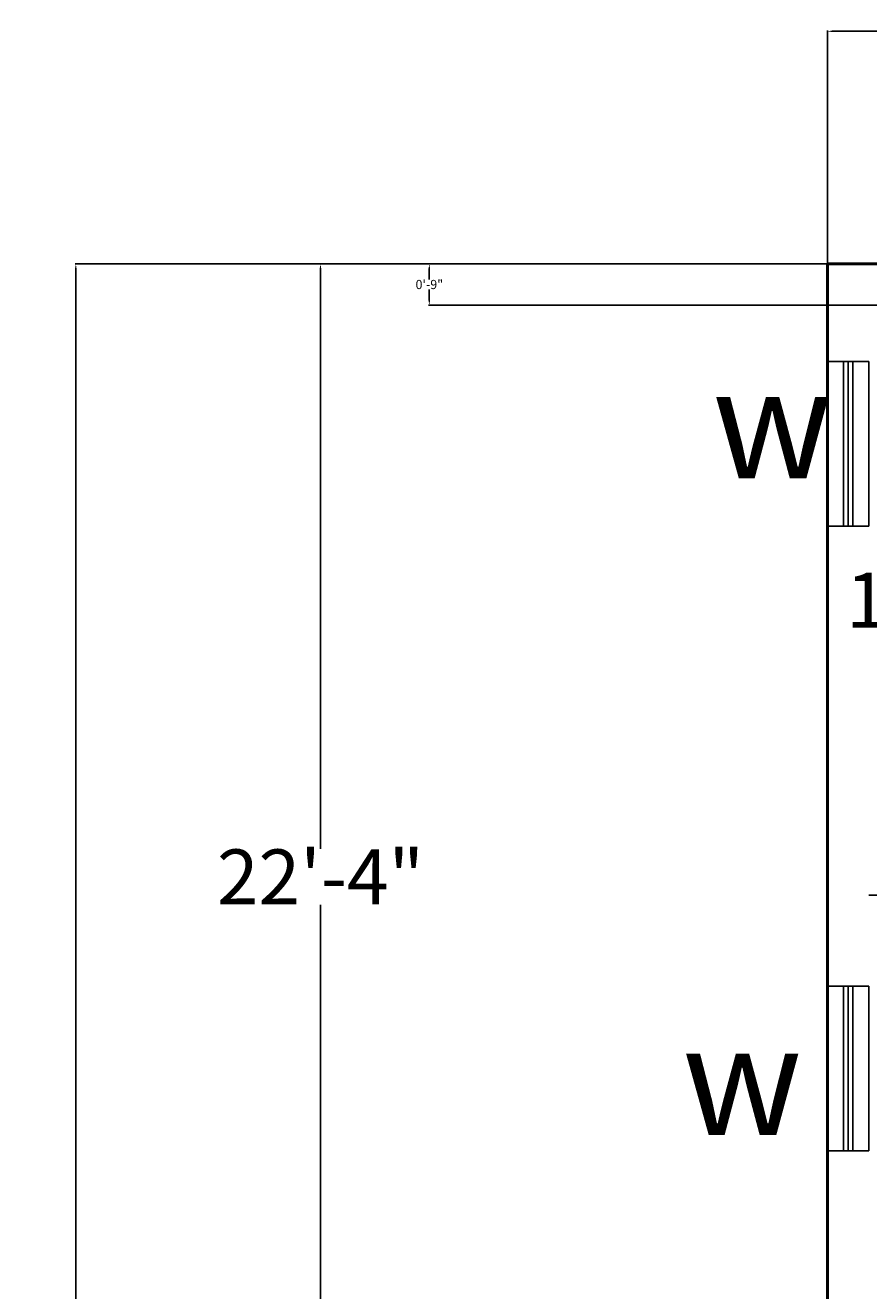
# Model space of a CAD drawing. Units: inches. Extents: x 409 to 7572, y 7 to 725.
# Tile 3 of 38: x 409 to 593, y 448 to 725. Entities that reach past the tile are written whole.
import ezdxf

# ---------------------------------------------------------------- set-up
doc = ezdxf.new("R2010")
doc.units = ezdxf.units.IN
doc.header["$MEASUREMENT"] = 0
for name, color, linetype, lineweight in [('A-ANNO-DIMS', 2, 'Continuous', 18), ('A-ANNO-SYMB', 3, 'Continuous', 25), ('A-GLAZ', 4, 'Continuous', 25), ('A-WALL', 7, 'Continuous', 50)]:
    doc.layers.add(name, color=color, linetype=linetype, lineweight=lineweight)
doc.styles.get("Standard").update_dxf_attribs({"font": 'arial.ttf'})
doc.dimstyles.get("Standard").update_dxf_attribs({"dimtxt": 2, "dimasz": 1, "dimexe": 0.18, "dimexo": 0.0625, "dimgap": 0.09, "dimtad": 0, "dimtih": 1, "dimtoh": 1, "dimdec": 0, "dimzin": 0, "dimdsep": 46, "dimlunit": 3, "dimtxsty": 'Standard', "dimcen": 0.09, "dimadec": 0, "dimazin": 0, "dimtfac": 1, "dimtdec": 0, "dimtofl": 0, "dimtmove": 0, "dimatfit": 3, "dimfxl": 1, "dimtolj": 1, "dimtzin": 0, "dimarcsym": 0})

# ---------------------------------------------------------------- blocks, each defined once
blk = doc.blocks.new('*D9')
at = {"layer": 'A-ANNO-DIMS', "color": 0, "lineweight": -2, "transparency": 16777216}
for p, q in [((593.22, 663.53), (610.99, 663.53)), ((610.81, 662.53), (610.81, 605.25)), ((610.81, 535.53), (610.81, 592.81)), ((593.22, 534.53), (610.99, 534.53))]:
    blk.add_line(p, q, dxfattribs=at)
at = {"layer": 'A-ANNO-DIMS', "color": 0, "transparency": 16777216}
for points in [[(610.64, 662.53), (610.98, 662.53), (610.81, 663.53)], [(610.64, 535.53), (610.98, 535.53), (610.81, 534.53)]]:
    blk.add_solid(points, dxfattribs=at)
at = {"layer": 'DEFPOINTS', "color": 0, "transparency": 16777216}
for p in [(593.16, 663.53), (593.16, 534.53), (610.81, 534.53)]:
    blk.add_point(p, dxfattribs=at)
at = {"layer": 'A-ANNO-DIMS', "color": 0, "transparency": 16777216, "insert": (610.81, 599.03), "char_height": 2, "attachment_point": 5}
blk.add_mtext('\\A1;{\\H6x;10\'-9"}', dxfattribs=at)
blk = doc.blocks.new('*D30')
at = {"layer": 'A-ANNO-DIMS', "color": 0, "lineweight": -2, "transparency": 16777216}
for p, q in [((584.16, 672.59), (584.16, 723.56)), ((585.16, 723.38), (851.59, 723.38)), ((1125.16, 723.38), (858.72, 723.38)), ((1126.16, 672.59), (1126.16, 723.56))]:
    blk.add_line(p, q, dxfattribs=at)
at = {"layer": 'A-ANNO-DIMS', "color": 0, "transparency": 16777216}
for points in [[(585.16, 723.55), (585.16, 723.22), (584.16, 723.38)], [(1125.16, 723.55), (1125.16, 723.22), (1126.16, 723.38)]]:
    blk.add_solid(points, dxfattribs=at)
at = {"layer": 'DEFPOINTS', "color": 0, "transparency": 16777216}
for p in [(584.16, 723.38), (584.16, 672.53), (1126.16, 672.53)]:
    blk.add_point(p, dxfattribs=at)
at = {"layer": 'A-ANNO-DIMS', "color": 0, "transparency": 16777216, "insert": (855.16, 723.38), "char_height": 2, "attachment_point": 5}
blk.add_mtext('\\A1;45\'-2"', dxfattribs=at)
blk = doc.blocks.new('*D31')
at = {"layer": 'A-ANNO-DIMS', "color": 0, "lineweight": -2, "transparency": 16777216}
for p, q in [((584.09, 672.53), (473.2, 672.53)), ((473.38, 671.53), (473.38, 544.65)), ((473.38, 405.53), (473.38, 532.42)), ((584.09, 404.53), (473.2, 404.53))]:
    blk.add_line(p, q, dxfattribs=at)
at = {"layer": 'A-ANNO-DIMS', "color": 0, "transparency": 16777216}
for points in [[(473.21, 671.53), (473.54, 671.53), (473.38, 672.53)], [(473.21, 405.53), (473.54, 405.53), (473.38, 404.53)]]:
    blk.add_solid(points, dxfattribs=at)
at = {"layer": 'DEFPOINTS', "color": 0, "transparency": 16777216}
for p in [(584.16, 672.53), (473.38, 404.53), (584.16, 404.53)]:
    blk.add_point(p, dxfattribs=at)
at = {"layer": 'A-ANNO-DIMS', "color": 0, "transparency": 16777216, "insert": (473.38, 538.53), "char_height": 2, "attachment_point": 5}
blk.add_mtext('\\A1;{\\H6x;22\'-4"}', dxfattribs=at)
blk = doc.blocks.new('*D34')
at = {"layer": 'A-ANNO-DIMS', "color": 0, "lineweight": -2, "transparency": 16777216}
for p, q in [((584.09, 672.53), (419.74, 672.53)), ((419.92, 671.53), (419.92, 420.75)), ((419.92, 157.53), (419.92, 408.31)), ((584.09, 156.53), (419.74, 156.53))]:
    blk.add_line(p, q, dxfattribs=at)
at = {"layer": 'A-ANNO-DIMS', "color": 0, "transparency": 16777216}
for points in [[(419.75, 671.53), (420.09, 671.53), (419.92, 672.53)], [(419.75, 157.53), (420.09, 157.53), (419.92, 156.53)]]:
    blk.add_solid(points, dxfattribs=at)
at = {"layer": 'DEFPOINTS', "color": 0, "transparency": 16777216}
for p in [(584.16, 672.53), (419.92, 156.53), (584.16, 156.53)]:
    blk.add_point(p, dxfattribs=at)
at = {"layer": 'A-ANNO-DIMS', "color": 0, "transparency": 16777216, "insert": (419.92, 414.53), "char_height": 2, "attachment_point": 5}
blk.add_mtext("\\A1;{\\H6x;43'}", dxfattribs=at)
blk = doc.blocks.new('WIN-36')
for p, q in [((1699.82, 514.65), (1699.82, 478.65)), ((1700.82, 514.65), (1700.82, 478.65)), ((1701.82, 514.65), (1701.82, 478.65))]:
    blk.add_line(p, q)
blk.add_lwpolyline([(1705.32, 514.65), (1705.32, 478.65), (1696.32, 478.65), (1696.32, 514.65)], close=True)
blk = doc.blocks.new('*D173')
at = {"layer": 'A-ANNO-DIMS', "color": 0, "lineweight": -2, "transparency": 16777216}
for p, q in [((584.09, 672.53), (496.98, 672.53)), ((497.16, 671.53), (497.16, 669.14)), ((497.16, 664.53), (497.16, 666.92)), ((593.09, 663.53), (496.98, 663.53))]:
    blk.add_line(p, q, dxfattribs=at)
at = {"layer": 'A-ANNO-DIMS', "color": 0, "transparency": 16777216}
for points in [[(496.99, 671.53), (497.32, 671.53), (497.16, 672.53)], [(496.99, 664.53), (497.32, 664.53), (497.16, 663.53)]]:
    blk.add_solid(points, dxfattribs=at)
at = {"layer": 'DEFPOINTS', "color": 0, "transparency": 16777216}
for p in [(584.16, 672.53), (497.16, 663.53), (593.16, 663.53)]:
    blk.add_point(p, dxfattribs=at)
at = {"layer": 'A-ANNO-DIMS', "color": 0, "transparency": 16777216, "insert": (497.16, 668.03), "char_height": 2, "attachment_point": 5}
blk.add_mtext('\\A1;0\'-9"', dxfattribs=at)

msp = doc.modelspace()

# ---------------------------------------------------------------- linework, layer by layer
at = {"layer": 'A-WALL'}
for p, q in [((1126.16, 672.53), (584.16, 672.53)), ((584.16, 672.53), (584.16, 404.53))]:
    msp.add_line(p, q, dxfattribs=at)

# ---------------------------------------------------------------- block references
at = {"layer": 'A-GLAZ'}
for p in [(-1112.16, 136.58), (-1112.16, 0)]:
    msp.add_blockref('WIN-36', p, dxfattribs=at)

# ---------------------------------------------------------------- texts
at = {"layer": 'A-ANNO-SYMB', "char_height": 24, "attachment_point": 1}
for insert in [(558.95, 649.67), (552.38, 506.09)]:
    msp.add_mtext_dynamic_manual_height_columns('w', width=18.2582, gutter_width=1, heights=[0], dxfattribs=dict(at, insert=insert))

# ---------------------------------------------------------------- dimensions: what is measured, and where the dimension line sits
at = {"layer": 'A-ANNO-DIMS'}
dim = msp.add_linear_dim(base=(584.16, 723.38), p1=(1126.16, 672.53), p2=(584.16, 672.53), dimstyle='Standard', override={"dimclrd": 0, "dimclre": 0, "dimclrt": 0}, dxfattribs=at)
dim.commit()
dim.dimension.update_dxf_attribs({"geometry": '*D30', "text_midpoint": (855.16, 723.38)})
for base, p1, p2, picture, middle in [((419.92, 156.53), (584.16, 672.53), (584.16, 156.53), '*D34', (419.92, 414.53)), ((473.38, 404.53), (584.16, 672.53), (584.16, 404.53), '*D31', (473.38, 538.53)), ((610.81, 534.53), (593.16, 663.53), (593.16, 534.53), '*D9', (610.81, 599.03))]:
    dim = msp.add_linear_dim(base=base, p1=p1, p2=p2, angle=90, text='{\\H6x;<>}', dimstyle='Standard', override={"dimclrd": 0, "dimclre": 0, "dimclrt": 0}, dxfattribs=at)
    dim.commit()
    dim.dimension.update_dxf_attribs({"geometry": picture, "text_midpoint": middle})
dim = msp.add_linear_dim(base=(497.16, 663.53), p1=(584.16, 672.53), p2=(593.16, 663.53), angle=90, dimstyle='Standard', override={"dimdec": 1, "dimlfac": 1, "dimrnd": 0, "dimzin": 1, "dimdsep": 46, "dimlunit": 4, "dimfrac": 2}, dxfattribs=at)
dim.commit()
dim.dimension.update_dxf_attribs({"geometry": '*D173', "text_midpoint": (497.16, 668.03)})

doc.saveas('drawing.dxf')
